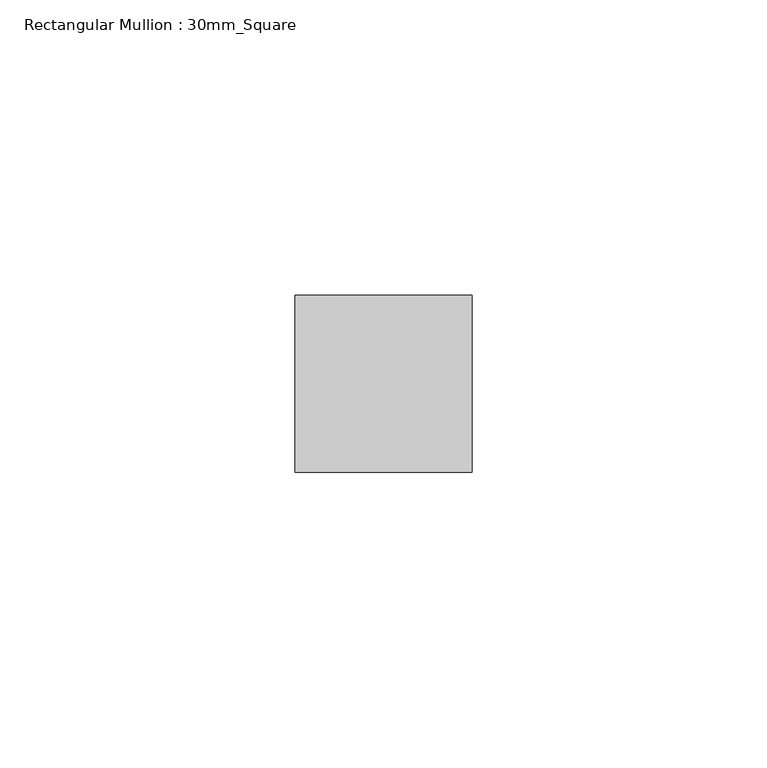
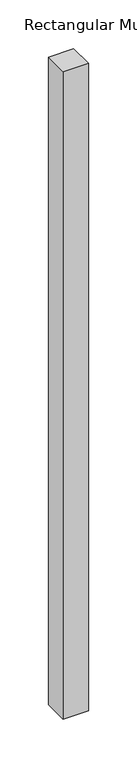
"""IFC4 building model written with IfcOpenShell, lengths in millimetres: member geometry, Rectangular Mullion : 30mm_Square."""

from ifc_helpers import new_model, si_unit, frame, origin, place, context, project, spatial, polyline, outline, extrude, source, transform, mapped, element, save


def rectangular_mullion_30mm_square_b0565101(model_context):
    return source(origin(), model_context, "Body", "SweptSolid", [
        extrude(outline(polyline([(0.0, 15.0), (0.0, -15.0), (-30.0, -15.0), (-30.0, 15.0), (0.0, 15.0)])), frame((0.0, 0.0, -812.9157956), z_axis=(0.0, 0.0, 1.0), x_axis=(1.0, 0.0, 0.0)), (0.0, 0.0, 1.0), 812.9157956),
    ])


if __name__ == "__main__":
    model = new_model("IFC4")
    model_context = context("Model", 3, world=origin())
    ifc_project = project(units=[si_unit("LENGTHUNIT", "METRE", prefix="MILLI")], contexts=[model_context])
    site = spatial("IfcSite", under=ifc_project)
    building = spatial("IfcBuilding", under=site)
    placement = place(None, origin())
    rectangular_mullion_30mm_square_shape = rectangular_mullion_30mm_square_b0565101(model_context)
    element("IfcMember", 1, ObjectType="Rectangular Mullion : 30mm_Square", at=placement, inside=building, context=model_context, shape_type="MappedRepresentation", body=[
        mapped(rectangular_mullion_30mm_square_shape, transform((0.0, 0.0, 0.0), x_axis=(1.0, 0.0, 0.0), y_axis=(0.0, 1.0, 0.0), z_axis=(0.0, 0.0, 1.0))),
    ])
    save(model, "model.ifc")

# Revit data of these elements
# Type "Rectangular Mullion : 30mm_Square"
#   Keynote = "H11"
#   built-in parameter 1007304 = 0.0984252 (stored number, unit not read)
#   built-in parameter 1007301 = 0.0492126 (stored number, unit not read)
#   built-in parameter 1007300 = 0.0492126 (stored number, unit not read)
# Element 1 (IfcMember, "Rectangular Mullion : 30mm_Square")
#   Materials on its faces: "Aluminium"
# Materials
#   "Aluminium": class "Metal", colour RGB 247 247 247, transparency 0, Description = "Aluminium 6061", Cost = 0
